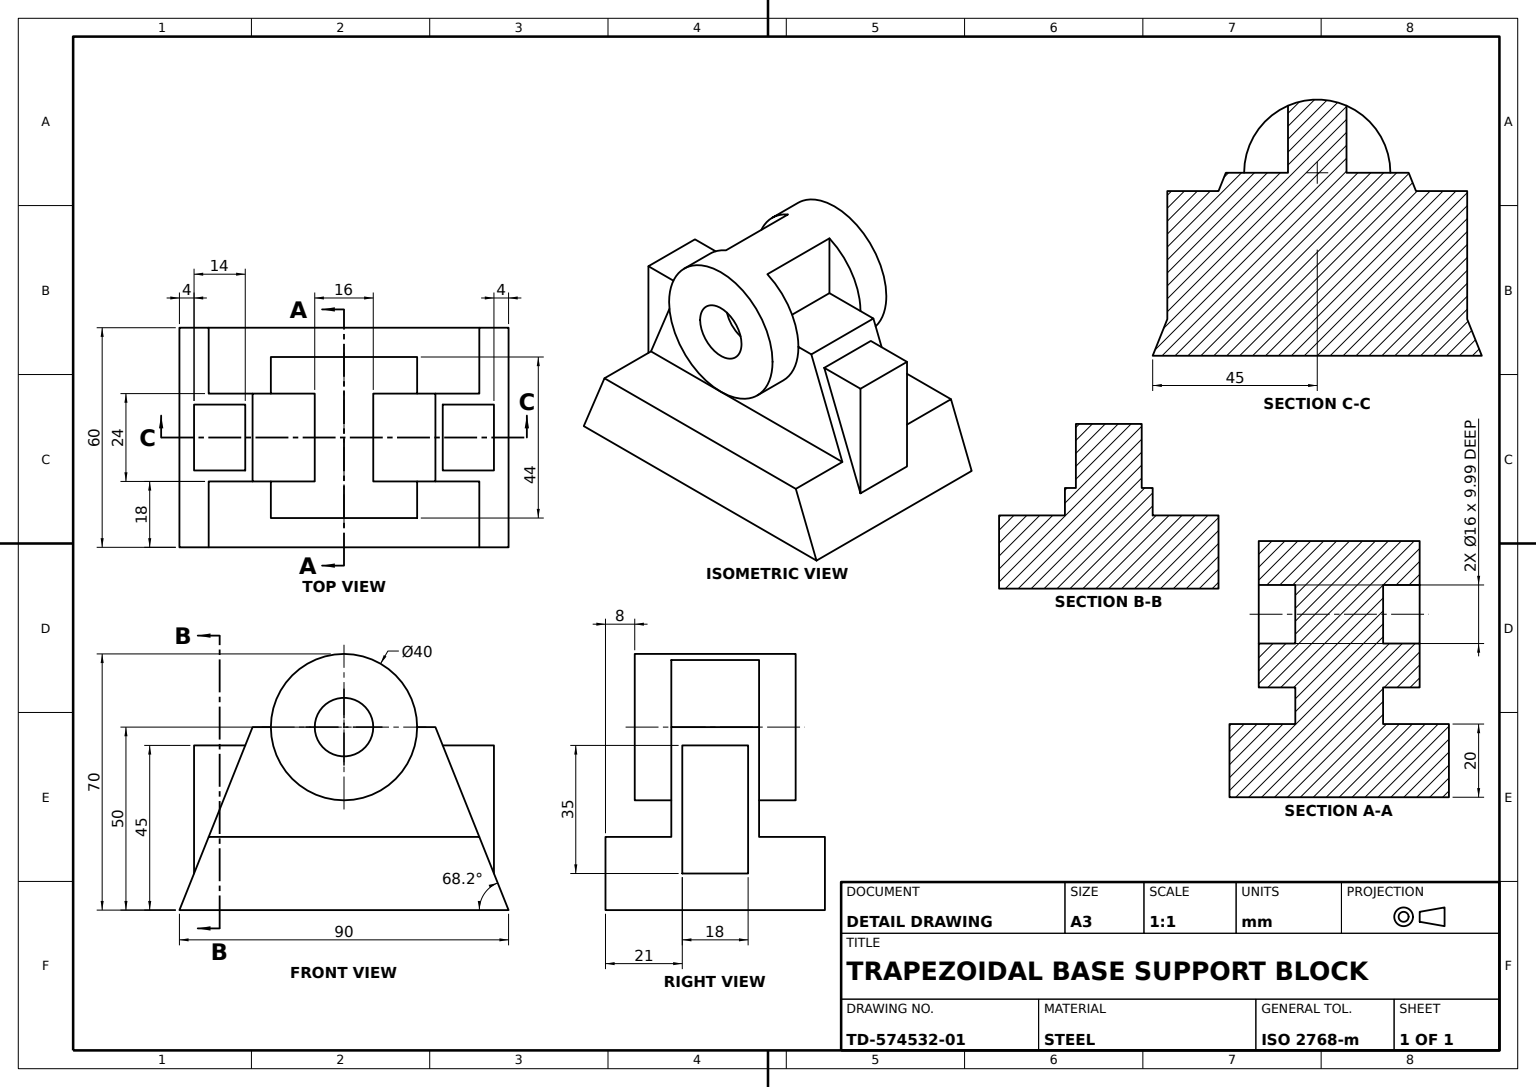
from build123d import *

# Parameters (mm, degrees)
BASE_BODY_DEPTH         = 30
SIDE_START              = -30
SIDE_POCKET_CUT_1_DEPTH = 18
SIDE_START_2            = 30
SIDE_POCKET_CUT_2_DEPTH = 18
SIDE_BLOCK_SKETCH_W     = 82
SIDE_BLOCK_SKETCH_H     = 35
SIDE_BLOCK_45X35_DEPTH  = 9
PIVOT_CYLINDER_SKETCH_R = 20
PIVOT_CYLINDER_40_DEPTH = 22
CYLINDER_SLOT_CUT_DEPTH = 12
PIVOT_BORE_SKETCH_R     = 8
PIVOT_BORE_16_DEPTH     = 9.99


with BuildPart() as part:
    # Base Profile Sketch → Base Body (new, symmetric)
    with BuildSketch(Plane(origin=(0, 0, 0), x_dir=(0, 0, -1), z_dir=(1, 0, 0))):
        Polygon((-45, 0), (45, 0), (25, 50), (0, 50), (-25, 50), align=None)
    extrude(amount=BASE_BODY_DEPTH, both=True)

    # Side Pocket Sketch → Side Pocket Cut 1 (cut)
    with BuildSketch(Plane(origin=(0, 0, 0), x_dir=(0, 0, -1), z_dir=(1, 0, 0)).offset(SIDE_START)):
        Polygon((-37, 20), (37, 20), (25, 50), (-25, 50), align=None)
    extrude(amount=SIDE_POCKET_CUT_1_DEPTH, mode=Mode.SUBTRACT)

    # Sketch5_2 → Side Pocket Cut 2 (cut)
    with BuildSketch(Plane(origin=(0, 0, 0), x_dir=(0, 0, -1), z_dir=(1, 0, 0)).offset(SIDE_START_2)):
        Polygon((-37, 20), (37, 20), (25, 50), (-25, 50), align=None)
    extrude(amount=-SIDE_POCKET_CUT_2_DEPTH, mode=Mode.SUBTRACT)

    # Side Block Sketch → Side Block 45x35 (add, symmetric)
    with BuildSketch(Plane(origin=(0, 0, 0), x_dir=(0, 0, -1), z_dir=(1, 0, 0))):
        with Locations((0, 27.5)):
            Rectangle(SIDE_BLOCK_SKETCH_W, SIDE_BLOCK_SKETCH_H)
    extrude(amount=SIDE_BLOCK_45X35_DEPTH, both=True)

    # Pivot Cylinder Sketch → Pivot Cylinder _40 (add, symmetric)
    with BuildSketch(Plane(origin=(0, 0, 0), x_dir=(0, 0, -1), z_dir=(1, 0, 0))):
        with Locations((0, 50)):
            Circle(PIVOT_CYLINDER_SKETCH_R)
    extrude(amount=PIVOT_CYLINDER_40_DEPTH, both=True)

    # Cylinder Slot Sketch → Cylinder Slot Cut (cut, symmetric)
    with BuildSketch(Plane(origin=(0, 0, 0), x_dir=(0, 0, -1), z_dir=(1, 0, 0))):
        with BuildLine():
            Line((-8, 68.33030278), (-8, 50))
            Line((-8, 50), (-20, 50))
            ThreePointArc((-20, 50), (-16.733200531, 60.95445115), (-8, 68.33030278))
        make_face()
    cylinder_slot_cut = extrude(amount=CYLINDER_SLOT_CUT_DEPTH, both=True, mode=Mode.SUBTRACT)

    # Cylinder Slot Mirror: Cylinder Slot Cut across plane
    add(cylinder_slot_cut.mirror(Plane.XY), mode=Mode.SUBTRACT)

    # Pivot Bore Sketch → Pivot Bore _16 (cut)
    with BuildSketch(Plane(origin=(22, 0, 0), x_dir=(0, 0, -1), z_dir=(1, 0, 0))):
        with Locations((0, 50)):
            Circle(PIVOT_BORE_SKETCH_R)
    pivot_bore_16 = extrude(amount=-PIVOT_BORE_16_DEPTH, mode=Mode.SUBTRACT)

    # Pivot Bore Mirror: Pivot Bore _16 across plane
    add(pivot_bore_16.mirror(Plane(origin=(0, 0, 0), x_dir=(0, 0, 1), z_dir=(1, 0, 0))), mode=Mode.SUBTRACT)


solid = part.part
